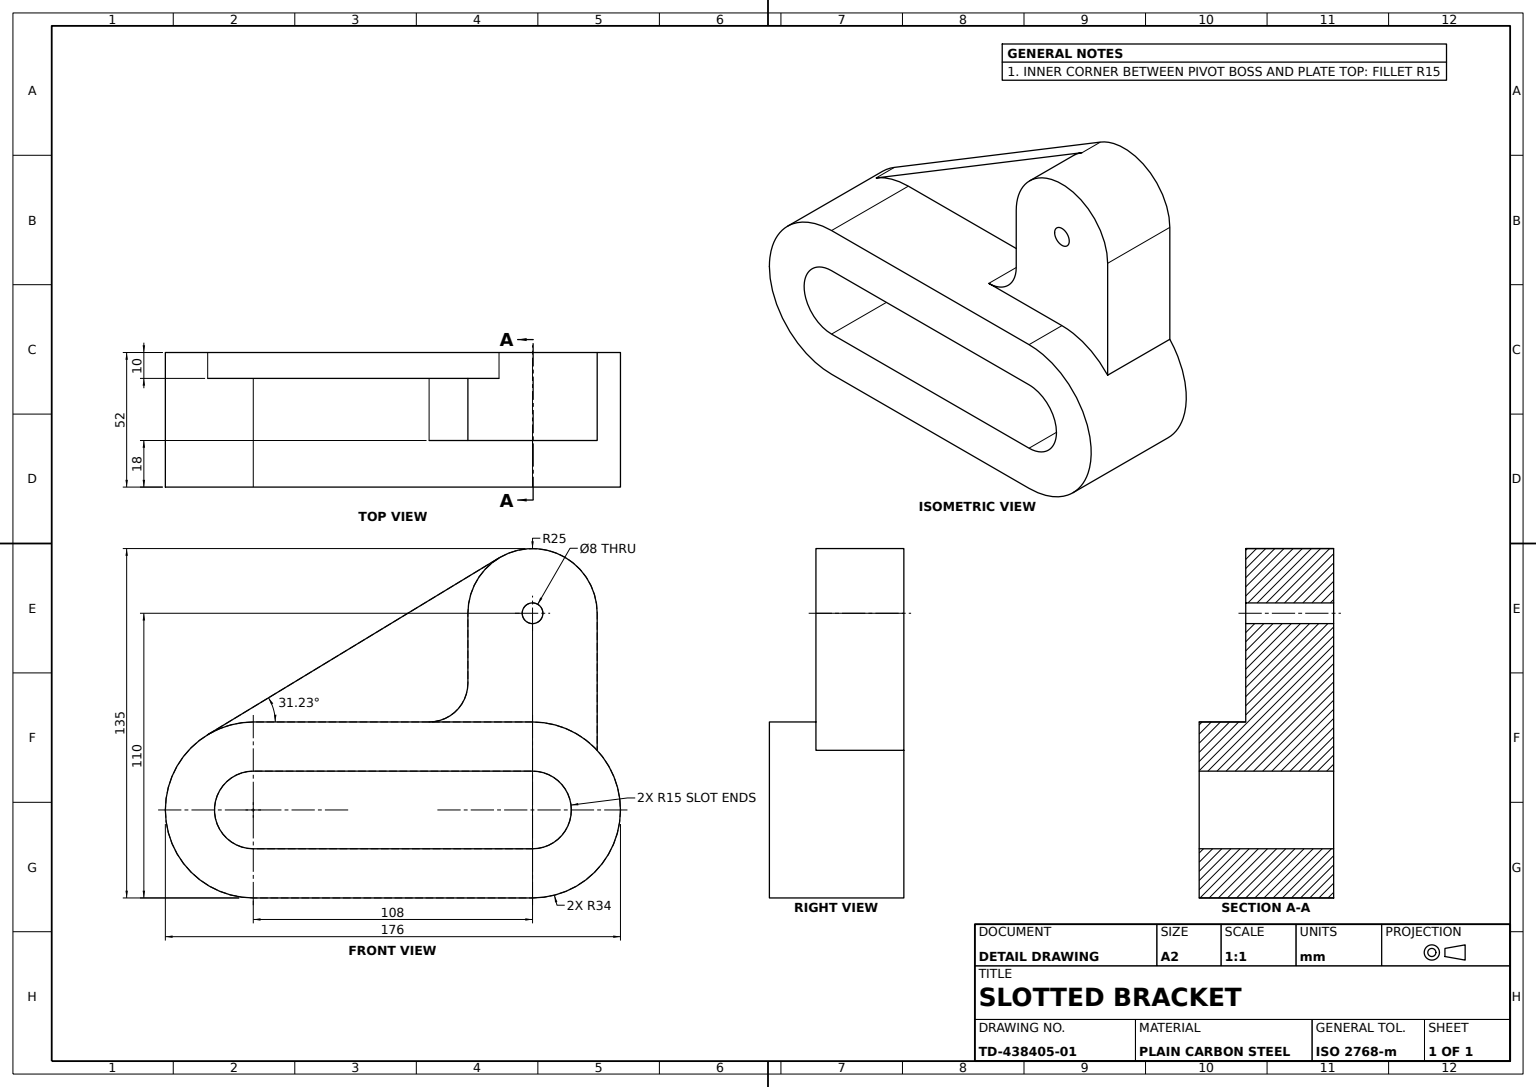
from build123d import *

# Parameters (mm, degrees)
LINK_PLATE_DEPTH          = 52
LINK_SLOT_DEPTH           = 52
PIVOT_BOSS_DEPTH          = 34
PIVOT_PIN_HOLE_SKETCH_R   = 4
PIVOT_PIN_HOLE_DEPTH      = 34
SUPPORT_RIB_10MM_REACH    = 145.698
SUPPORT_RIB_SKETCH_WALL_W = 421.148756116
SUPPORT_RIB_SKETCH_WALL_H = 10
EDGE_FILLETS_R15_R        = 15


with BuildPart() as part:
    # Link Plate Outline Sketch → Link Plate (new body)
    with BuildSketch(Plane.XY):
        with BuildLine():
            Line((-54, 34), (54, 34))
            ThreePointArc((54, 34), (88, 0), (54, -34))
            Line((54, -34), (-54, -34))
            ThreePointArc((-54, -34), (-88, 0), (-54, 34))
        make_face()
    extrude(amount=LINK_PLATE_DEPTH)

    # Link Slot Sketch → Link Slot (cut)
    with BuildSketch(Plane.XY.offset(52)):
        with BuildLine():
            Line((-54, 15), (54, 15))
            ThreePointArc((54, 15), (69, 0), (54, -15))
            Line((54, -15), (-54, -15))
            ThreePointArc((-54, -15), (-69, 0), (-54, 15))
        make_face()
    extrude(amount=-LINK_SLOT_DEPTH, mode=Mode.SUBTRACT)

    # Pivot Boss Sketch → Pivot Boss (add)
    with BuildSketch(Plane.XY):
        with BuildLine():
            Line((29, 76), (29, 34))
            Line((29, 34), (29, 18.031591918))
            Line((29, 18.031591918), (79, 18.031591918))
            Line((79, 18.031591918), (79, 76))
            ThreePointArc((79, 76), (54, 101), (29, 76))
        make_face()
    extrude(amount=PIVOT_BOSS_DEPTH)

    # Pivot Pin Hole Sketch → Pivot Pin Hole (cut)
    with BuildSketch(Plane.XY.offset(34)):
        with Locations((54, 76)):
            Circle(PIVOT_PIN_HOLE_SKETCH_R)
    extrude(amount=-PIVOT_PIN_HOLE_DEPTH, mode=Mode.SUBTRACT)

    # Support Rib Sketch wall → Support Rib 10mm (add, up to next)
    with BuildSketch(Plane(origin=(-15.293433294, 63.226194681, 0), x_dir=(0.855125243419, 0.518421467599, 0), z_dir=(-0.518421467599, 0.855125243419, 0)), mode=Mode.PRIVATE) as support_rib_10mm_sk1:
        with Locations((0, -5)):
            Rectangle(SUPPORT_RIB_SKETCH_WALL_W, SUPPORT_RIB_SKETCH_WALL_H)
    support_rib_10mm_tool1 = extrude(support_rib_10mm_sk1.sketch, amount=-SUPPORT_RIB_10MM_REACH, mode=Mode.PRIVATE) - part.part
    add(support_rib_10mm_tool1.solids().sort_by_distance((-15.293433294, 63.226194681, 0))[0])

    # Edge Fillets R15
    edge_fillets_r15_edges = [part.edges().sort_by_distance(p)[0] for p in [
        (29, 34, 22),
    ]]
    fillet(edge_fillets_r15_edges, radius=EDGE_FILLETS_R15_R)


solid = part.part
